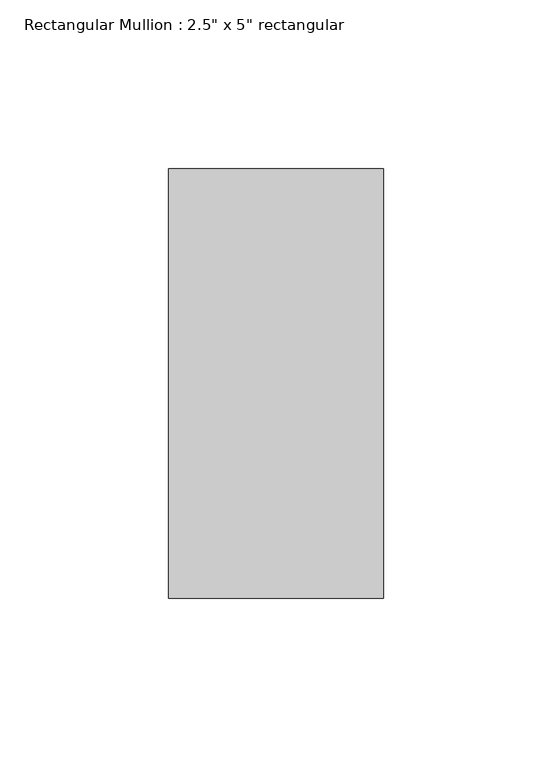
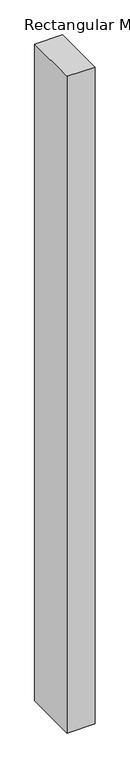
"""IFC4 building model written with IfcOpenShell, lengths in millimetres: member geometry."""

from ifc_helpers import new_model, si_unit, frame, origin, place, context, project, spatial, polyline, outline, extrude, source, transform, mapped, element, save


def member_6b6fe981(model_context):
    return source(origin(), model_context, "Body", "SweptSolid", [
        extrude(outline(polyline([(0.0, 63.5), (0.0, -63.5), (-63.5, -63.5), (-63.5, 63.5), (0.0, 63.5)])), frame((0.0, 0.0, -1569.7635787), z_axis=(0.0, 0.0, 1.0), x_axis=(1.0, 0.0, 0.0)), (0.0, 0.0, 1.0), 1569.7635787),
    ])


if __name__ == "__main__":
    model = new_model("IFC4")
    model_context = context("Model", 3, world=origin())
    ifc_project = project(units=[si_unit("LENGTHUNIT", "METRE", prefix="MILLI")], contexts=[model_context])
    site = spatial("IfcSite", under=ifc_project)
    building = spatial("IfcBuilding", under=site)
    placement = place(None, origin())
    member_shape = member_6b6fe981(model_context)
    element("IfcMember", 1, ObjectType="Rectangular Mullion : 2.5\" x 5\" rectangular", at=placement, inside=building, context=model_context, shape_type="MappedRepresentation", body=[
        mapped(member_shape, transform((0.0, 0.0, 0.0), x_axis=(1.0, 0.0, 0.0), y_axis=(0.0, 1.0, 0.0), z_axis=(0.0, 0.0, 1.0))),
    ])
    save(model, "model.ifc")

# Revit data of these elements
# Type "Rectangular Mullion : 2.5\" x 5\" rectangular"
#   built-in parameter 1007304 = 0.416667 (stored number, unit not read)
#   built-in parameter 1007301 = 0.104167 (stored number, unit not read)
#   built-in parameter 1007300 = 0.104167 (stored number, unit not read)
# Element 1 (IfcMember, "Rectangular Mullion : 2.5\" x 5\" rectangular")
#   Materials on its faces: "Aluminum"
# Materials
#   "Aluminum": class "Metal", colour RGB 247 247 247, transparency 0, Description = "Aluminum 6061", Cost = 0
